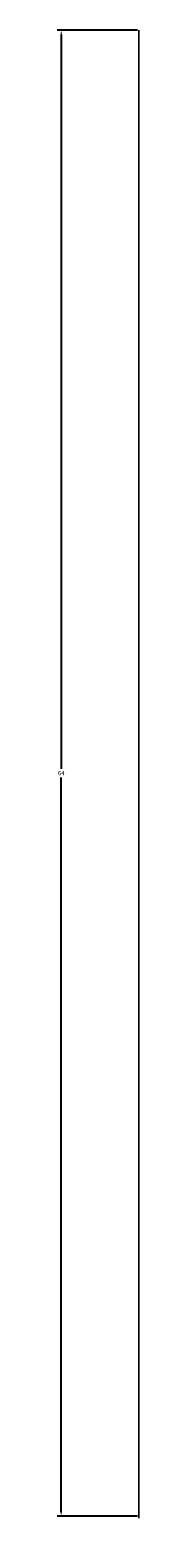
# Model space of a CAD drawing. Units: millimetres. Extents: x -4 to 2856, y -2 to 1373.
# Tile 1 of 3: x -4 to 0, y 1308 to 1373. Entities that reach past the tile are written whole.
import ezdxf

# ---------------------------------------------------------------- set-up
doc = ezdxf.new("R2010")
doc.units = ezdxf.units.MM
doc.layers.add('M-CONS', color=8, linetype='Continuous', lineweight=18)
doc.layers.add('M-DIMS', color=2, linetype='Continuous', lineweight=18)
doc.styles.get("Standard").update_dxf_attribs({"font": 'arial.ttf'})
doc.dimstyles.get("Standard").update_dxf_attribs({"dimtxt": 0.18, "dimasz": 0.18, "dimexe": 0.18, "dimexo": 0.0625, "dimgap": 0.09, "dimtad": 0, "dimtih": 1, "dimtoh": 1, "dimdec": 4, "dimzin": 0, "dimdsep": 46, "dimtxsty": 'Standard', "dimcen": 0.09, "dimadec": 0, "dimazin": 0, "dimtfac": 1, "dimtdec": 4, "dimtofl": 0, "dimtmove": 0, "dimatfit": 3, "dimfxl": 1, "dimtolj": 1, "dimtzin": 0, "dimarcsym": 0})

# ---------------------------------------------------------------- blocks, each defined once
blk = doc.blocks.new('*D6')
at = {"layer": 'Defpoints', "color": 0, "transparency": 16777216}
for p in [(-3.35, 1373.214), (0, 1373.214), (0, 1309.214)]:
    blk.add_point(p, dxfattribs=at)
at = {"layer": 'M-DIMS', "color": 0, "lineweight": -2, "transparency": 16777216}
for p, q in [((-0.062, 1373.214), (-3.53, 1373.214)), ((-3.35, 1373.034), (-3.35, 1341.396)), ((-3.35, 1309.394), (-3.35, 1341.032)), ((-0.062, 1309.214), (-3.53, 1309.214))]:
    blk.add_line(p, q, dxfattribs=at)
at = {"layer": 'M-DIMS', "color": 0, "transparency": 16777216}
for points in [[(-3.38, 1373.034), (-3.32, 1373.034), (-3.35, 1373.214)], [(-3.38, 1309.394), (-3.32, 1309.394), (-3.35, 1309.214)]]:
    blk.add_solid(points, dxfattribs=at)
at = {"layer": 'M-DIMS', "color": 0, "transparency": 16777216, "insert": (-3.35, 1341.214), "char_height": 0.18, "attachment_point": 5}
blk.add_mtext('\\A1;64', dxfattribs=at)

msp = doc.modelspace()

# ---------------------------------------------------------------- linework, layer by layer
at = {"layer": 'M-CONS', "extrusion": (1, 0, 0)}
msp.add_lwpolyline([(1373.214, 65.258, 0.536675), (1309.214, 17.258), (1309.214, 1.258), (1373.214, 1.258)], format="xyb", close=True, dxfattribs=at)

# ---------------------------------------------------------------- dimensions: what is measured, and where the dimension line sits
at = {"layer": 'M-DIMS'}
dim = msp.add_linear_dim(base=(-3.35, 1373.214), p1=(0, 1309.214), p2=(0, 1373.214), angle=90, dimstyle='Standard', override={"dimdec": 0, "dimlfac": 1, "dimrnd": 0, "dimzin": 0, "dimdsep": 46, "dimlunit": 2}, dxfattribs=at)
dim.commit()
dim.dimension.update_dxf_attribs({"geometry": '*D6', "text_midpoint": (-3.35, 1341.214)})

doc.saveas('drawing.dxf')
